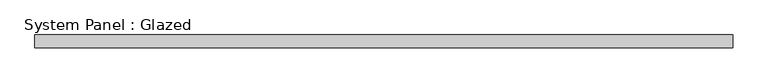
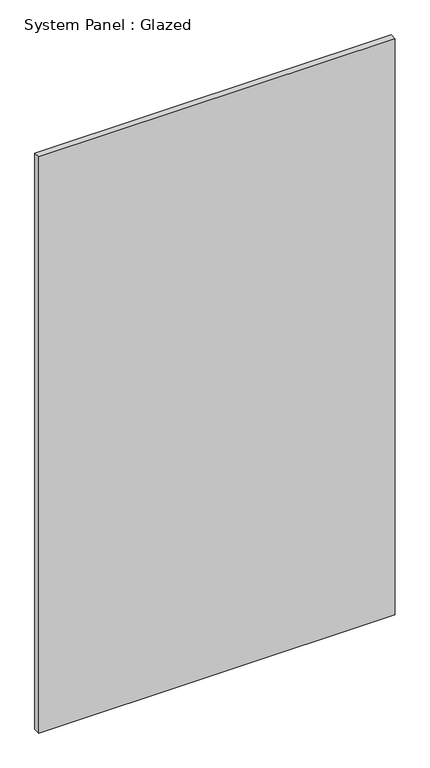
"""IFC4 building model written with IfcOpenShell, lengths in millimetres: plate geometry, System Panel : Glazed."""

from ifc_helpers import new_model, si_unit, origin, origin_with_axes, place, context, project, spatial, polyline, outline, extrude, source, transform, mapped, element, save


def system_panel_glazed_9f7cb957(model_context):
    return source(origin(), model_context, "Body", "SweptSolid", [
        extrude(outline(polyline([(685.7999999, 19.05), (-685.7999999, 19.05), (-685.7999999, 44.45), (685.7999999, 44.45), (685.7999999, 19.05)])), origin_with_axes(), (0.0, 0.0, 1.0), 2343.15),
    ])


if __name__ == "__main__":
    model = new_model("IFC4")
    model_context = context("Model", 3, world=origin())
    ifc_project = project(units=[si_unit("LENGTHUNIT", "METRE", prefix="MILLI")], contexts=[model_context])
    site = spatial("IfcSite", under=ifc_project)
    building = spatial("IfcBuilding", under=site)
    placement = place(None, origin())
    system_panel_glazed_shape = system_panel_glazed_9f7cb957(model_context)
    element("IfcPlate", 1, ObjectType="System Panel : Glazed", at=placement, inside=building, context=model_context, shape_type="MappedRepresentation", body=[
        mapped(system_panel_glazed_shape, transform((0.0, 0.0, 0.0), x_axis=(1.0, 0.0, 0.0), y_axis=(0.0, 1.0, 0.0), z_axis=(0.0, 0.0, 1.0))),
    ])
    save(model, "model.ifc")

# Revit data of these elements
# Type "System Panel : Glazed"
#   Construction Type Id = "GSP4R"
#   Analytic Construction = "1/8 in Pilkington single glazing"
#   Visual Light Transmittance = 0.9
#   Solar Heat Gain Coefficient = 0.86
#   Heat Transfer Coefficient (U) = 1.18115 BTU/(h·ft²·°F)
#   Define Thermal Properties by = 1
# Element 1 (IfcPlate, "System Panel : Glazed")
#   Materials on its faces: "Glass"
# Materials
#   "Glass": class "Glass", colour RGB 0 128 192, transparency 0.75, Description = "Soda Lime Glass", Cost = 0
